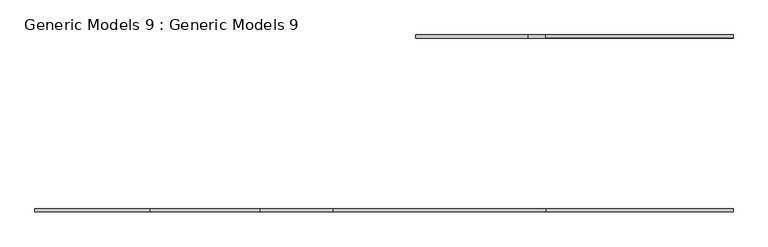
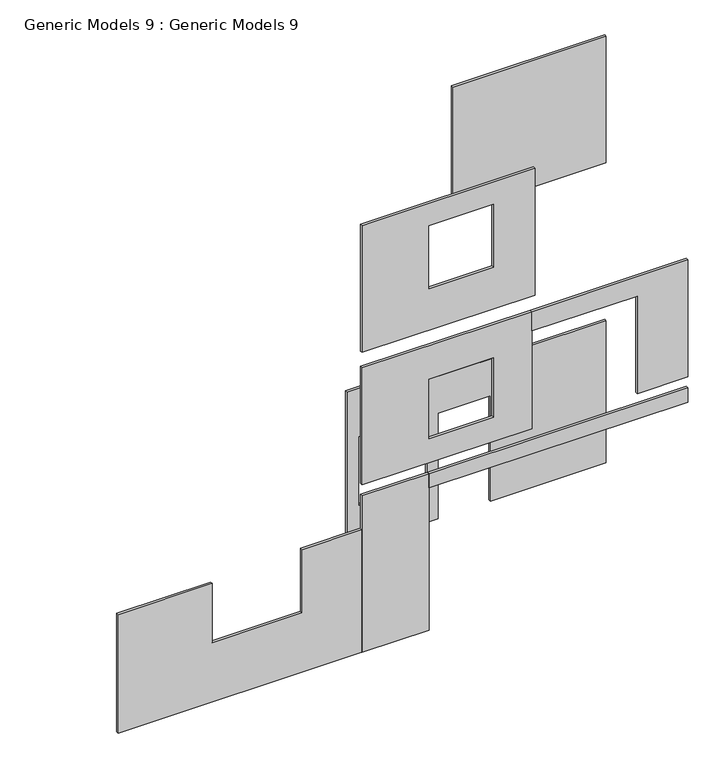
"""IFC4 building model written with IfcOpenShell, lengths in millimetres: proxy geometry, Generic Models 9 : Generic Models 9."""

from ifc_helpers import new_model, si_unit, frame, origin, origin_with_axes, place, context, project, spatial, polyline, outline, extrude, faceted_brep, source, transform, mapped, element, save


def generic_models_9_generic_models_9_83f75d2b(model_context):
    return source(origin(), model_context, "Body", "SolidModel", [
        extrude(outline(polyline([(3352.8, -9672.7398728), (3352.8, -11530.0195233), (0.0, -11530.0195233), (0.0, -9683.5057237), (2260.6, -9683.5057237), (2260.6, -8615.3695233), (0.0, -8615.3695233), (0.0, -6272.2195233), (3048.0, -6272.2195233), (3048.0, -9672.7398728), (3352.8, -9672.7398728)]), holes=[polyline([(2316.9077492, -11282.3695233), (2316.9077492, -9910.7695233), (844.8572576, -9910.7695233), (844.8572576, -11282.3695233), (2316.9077492, -11282.3695233)])]), frame((0.0, -11309.0252569, 0.0), z_axis=(0.0, 1.0, 0.0), x_axis=(0.0, 0.0, 1.0)), (0.0, 0.0, 1.0), 50.8),
        extrude(outline(polyline([(-6272.2195233, -14185.5752569), (-11530.0195233, -14185.5752569), (-11530.0195233, -14134.7752569), (-6272.2195233, -14134.7752569), (-6272.2195233, -14185.5752569)])), frame((0.0, 0.0, 3048.0), z_axis=(0.0, 0.0, 1.0), x_axis=(1.0, 0.0, 0.0)), (0.0, 0.0, 1.0), 304.8),
        extrude(outline(polyline([(6096.0, -6272.2195233), (6096.0, -9434.5195233), (5682.139627, -9434.5195233), (5682.139627, -7300.9195233), (3588.5355704, -7300.9195233), (3588.5355704, -6272.2195233), (6096.0, -6272.2195233)])), frame((0.0, -14185.5752569, 0.0), z_axis=(0.0, 1.0, 0.0), x_axis=(0.0, 0.0, 1.0)), (0.0, 0.0, 1.0), 50.8),
        extrude(outline(polyline([(2540.9085414, -15930.5695233), (2540.9085414, -17832.2537599), (0.0, -17832.2537599), (0.0, -12892.4603585), (2626.8131853, -12892.4603585), (2626.8131853, -14101.7695233), (1270.940225, -14101.7695233), (1270.940225, -15930.5695233), (2540.9085414, -15930.5695233)])), frame((0.0, -14185.5752569, 0.0), z_axis=(0.0, 1.0, 0.0), x_axis=(0.0, 0.0, 1.0)), (0.0, 0.0, 1.0), 50.8),
        extrude(outline(polyline([(-11530.0195233, -14185.5752569), (-12886.9719936, -14185.5752569), (-12886.9719936, -14134.7752569), (-11530.0195233, -14134.7752569), (-11530.0195233, -14185.5752569)])), origin_with_axes(), (0.0, 0.0, 1.0), 3352.8),
        extrude(outline(polyline([(3588.5355704, -9434.5195233), (6096.0, -9434.5195233), (6096.0, -12884.8411453), (3588.5355704, -12884.8411453), (3588.5355704, -9434.5195233)]), holes=[polyline([(5377.8228134, -10215.5695233), (4104.4168129, -10215.5695233), (4104.4168129, -11530.0195233), (5377.8228134, -11530.0195233), (5377.8228134, -10215.5695233)])]), frame((0.0, -14185.5752569, 0.0), z_axis=(0.0, 1.0, 0.0), x_axis=(0.0, 0.0, 1.0)), (0.0, 0.0, 1.0), 50.8),
        extrude(outline(polyline([(-6272.2195233, -11309.0252569), (-9377.3695233, -11309.0252569), (-9377.3695233, -11258.2252569), (-6272.2195233, -11258.2252569), (-6272.2195233, -11309.0252569)])), frame((0.0, 0.0, 6429.1436541), z_axis=(0.0, 0.0, 1.0), x_axis=(1.0, 0.0, 0.0)), (0.0, 0.0, 1.0), 2714.8563459),
        faceted_brep([(-9377.3695233, -14185.5752569, 9144.0), (-12889.5926394, -14185.5752569, 9144.0), (-12889.569466, -14185.5752569, 6429.1436541), (-9377.3695233, -14185.5752569, 6429.1436541), (-11530.0195233, -14185.5752569, 8672.741835), (-10215.5695233, -14185.5752569, 8672.741835), (-10215.5695233, -14185.5752569, 7322.7664741), (-11530.0195233, -14185.5752569, 7322.7664741), (-12889.569466, -14134.7752569, 6429.1436541), (-12889.5926394, -14134.7752569, 9144.0), (-9377.3695233, -14134.7752569, 9144.0), (-9377.3695233, -14134.7752569, 6429.1436541), (-11530.0195233, -14134.7752569, 7322.7664741), (-10215.5695233, -14134.7752569, 7322.7664741), (-10215.5695233, -14134.7752569, 8672.741835), (-11530.0195233, -14134.7752569, 8672.741835)], [[[0, 1, 2, 3], [4, 5, 6, 7]], [[8, 9, 10, 11], [12, 13, 14, 15]], [[8, 2, 1, 9]], [[3, 2, 8, 11]], [[15, 4, 7, 12]], [[1, 0, 10, 9]], [[4, 15, 14, 5]], [[0, 3, 11, 10]], [[7, 6, 13, 12]], [[6, 5, 14, 13]]]),
    ])


if __name__ == "__main__":
    model = new_model("IFC4")
    model_context = context("Model", 3, world=origin())
    ifc_project = project(units=[si_unit("LENGTHUNIT", "METRE", prefix="MILLI")], contexts=[model_context])
    site = spatial("IfcSite", under=ifc_project)
    building = spatial("IfcBuilding", under=site)
    placement = place(None, origin())
    generic_models_9_generic_models_9_shape = generic_models_9_generic_models_9_83f75d2b(model_context)
    element("IfcBuildingElementProxy", 1, Name="Generic Models 9 : Generic Models 9", ObjectType="Generic Models 9 : Generic Models 9", at=placement, inside=building, context=model_context, shape_type="MappedRepresentation", body=[
        mapped(generic_models_9_generic_models_9_shape, transform((0.0, 0.0, 0.0), x_axis=(1.0, 0.0, 0.0), y_axis=(0.0, 1.0, 0.0), z_axis=(0.0, 0.0, 1.0))),
    ])
    save(model, "model.ifc")
